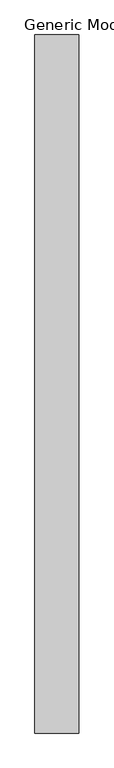
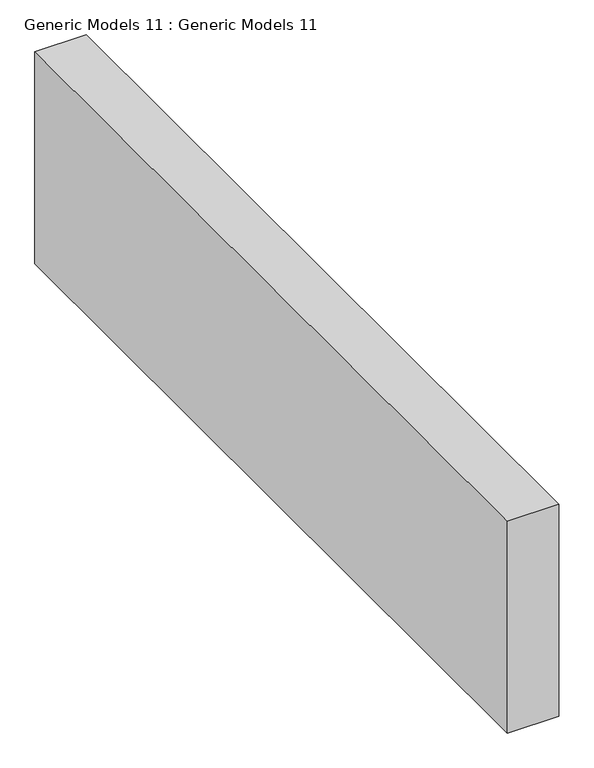
"""IFC4 building model written with IfcOpenShell, lengths in millimetres: proxy geometry, Generic Models 11 : Generic Models 11."""

from ifc_helpers import new_model, si_unit, frame, origin, place, context, project, spatial, polyline, outline, extrude, source, transform, mapped, element, save


def generic_models_11_generic_models_11_40482c90(model_context):
    return source(origin(), model_context, "Body", "SweptSolid", [
        extrude(outline(polyline([(-13072.9906521, -7693.1810793), (-13072.9906521, -5260.3016611), (-12920.5906521, -5260.3016611), (-12920.5906521, -7693.1810793), (-13072.9906521, -7693.1810793)])), frame((0.0, 0.0, 2540.0), z_axis=(0.0, 0.0, 1.0), x_axis=(1.0, 0.0, 0.0)), (0.0, 0.0, 1.0), 665.4216329),
    ])


if __name__ == "__main__":
    model = new_model("IFC4")
    model_context = context("Model", 3, world=origin())
    ifc_project = project(units=[si_unit("LENGTHUNIT", "METRE", prefix="MILLI")], contexts=[model_context])
    site = spatial("IfcSite", under=ifc_project)
    building = spatial("IfcBuilding", under=site)
    placement = place(None, origin())
    generic_models_11_generic_models_11_shape = generic_models_11_generic_models_11_40482c90(model_context)
    element("IfcBuildingElementProxy", 1, Name="Generic Models 11 : Generic Models 11", ObjectType="Generic Models 11 : Generic Models 11", at=placement, inside=building, context=model_context, shape_type="MappedRepresentation", body=[
        mapped(generic_models_11_generic_models_11_shape, transform((0.0, 0.0, 0.0), x_axis=(1.0, 0.0, 0.0), y_axis=(0.0, 1.0, 0.0), z_axis=(0.0, 0.0, 1.0))),
    ])
    save(model, "model.ifc")

# Revit data of these elements
# Element 1 (IfcBuildingElementProxy, "Generic Models 11 : Generic Models 11")
#   Materials on its faces: "GREY COLOUR FRAME(2)"
# Materials
#   "GREY COLOUR FRAME(2)": class "Generic", colour RGB 120 120 120, transparency 0, Cost = 0
